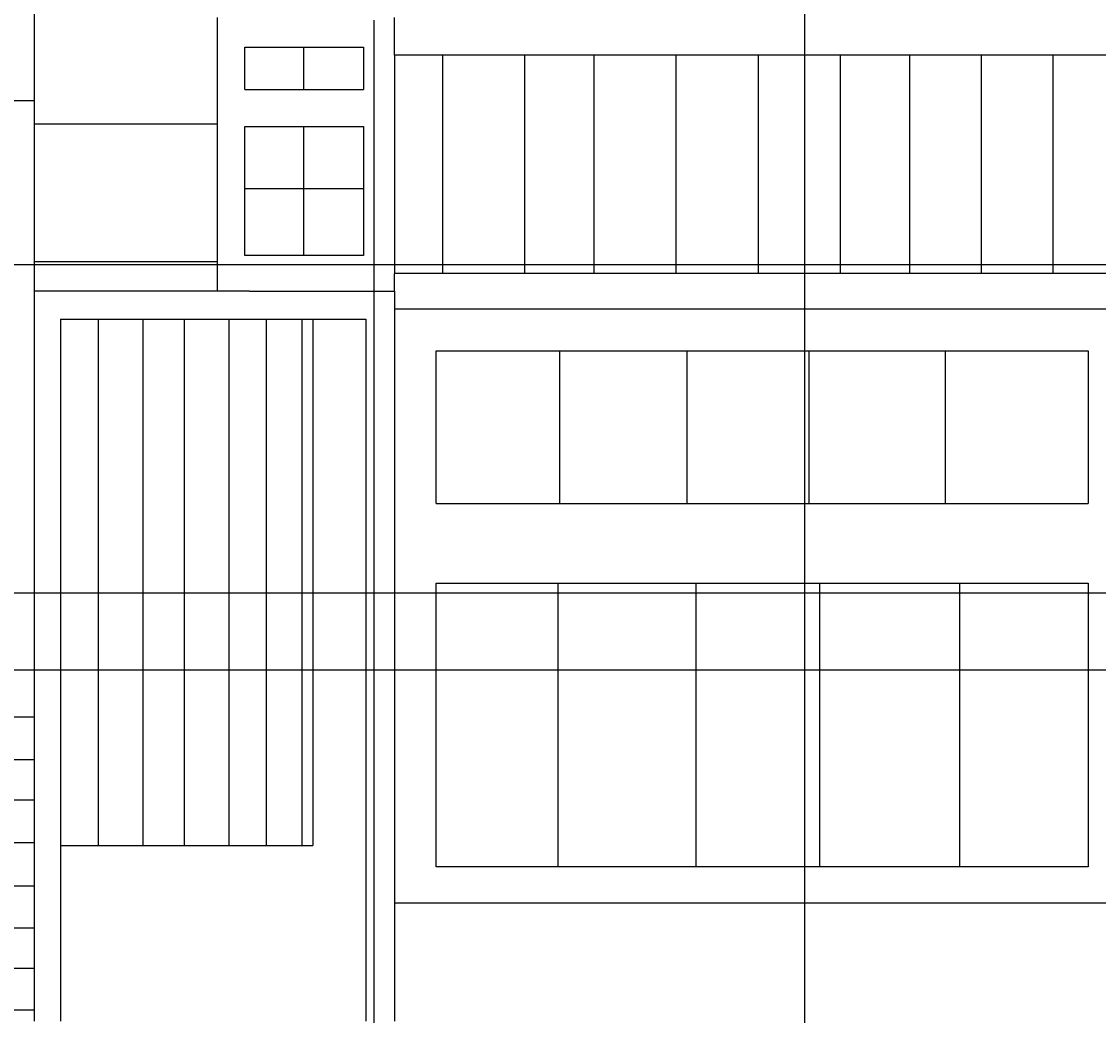
# Model space of a CAD drawing. Units: inches. Extents: x -117 to 121, y -77 to 40.
# Tile 21 of 45: x -23 to 3, y -32 to -8. Entities that reach past the tile are written whole.
import ezdxf

# ---------------------------------------------------------------- set-up
doc = ezdxf.new("R2010")
doc.units = ezdxf.units.IN
doc.header["$MEASUREMENT"] = 0
doc.layers.add('A-ANNO-DIMS', color=2, linetype='Continuous', lineweight=18)
doc.layers.add('A-ELEV', color=7, linetype='Continuous', lineweight=25)
doc.styles.get("Standard").update_dxf_attribs({"font": 'arial.ttf'})
doc.dimstyles.get("Standard").update_dxf_attribs({"dimtxt": 0.18, "dimasz": 0.18, "dimexe": 0.18, "dimexo": 0.0625, "dimgap": 0.09, "dimtad": 0, "dimtih": 1, "dimtoh": 1, "dimdec": 4, "dimzin": 0, "dimdsep": 46, "dimtxsty": 'Standard', "dimcen": 0.09, "dimadec": 0, "dimazin": 0, "dimtfac": 1, "dimtdec": 4, "dimtofl": 0, "dimtmove": 0, "dimatfit": 3, "dimfxl": 1, "dimtolj": 1, "dimtzin": 0, "dimarcsym": 0})

# ---------------------------------------------------------------- blocks, each defined once
blk = doc.blocks.new('*D13')
at = {"layer": 'A-ANNO-DIMS', "color": 0, "lineweight": -2, "transparency": 16777216}
for p, q in [((-2.663, 27.063), (-117.024, 27.063)), ((-116.844, 26.883), (-116.844, -16.974)), ((-116.844, -61.196), (-116.844, -17.338)), ((-106.096, -61.376), (-117.024, -61.376))]:
    blk.add_line(p, q, dxfattribs=at)
at = {"layer": 'A-ANNO-DIMS', "color": 0, "transparency": 16777216}
for points in [[(-116.874, 26.883), (-116.814, 26.883), (-116.844, 27.063)], [(-116.874, -61.196), (-116.814, -61.196), (-116.844, -61.376)]]:
    blk.add_solid(points, dxfattribs=at)
at = {"layer": 'Defpoints', "color": 0, "transparency": 16777216}
for p in [(-2.6, 27.063), (-116.844, -61.376), (-106.034, -61.376)]:
    blk.add_point(p, dxfattribs=at)
at = {"layer": 'A-ANNO-DIMS', "color": 0, "transparency": 16777216, "insert": (-116.844, -17.156), "char_height": 0.18, "attachment_point": 5}
blk.add_mtext('\\A1;88.44', dxfattribs=at)
blk = doc.blocks.new('*D32')
at = {"layer": 'A-ANNO-DIMS', "color": 0, "lineweight": -2, "transparency": 16777216}
for p, q in [((-3.85, -45.55), (-3.85, 38.61)), ((-3.67, 38.43), (7.757, 38.43)), ((20.113, 38.43), (8.686, 38.43)), ((20.293, -45.55), (20.293, 38.61))]:
    blk.add_line(p, q, dxfattribs=at)
at = {"layer": 'A-ANNO-DIMS', "color": 0, "transparency": 16777216}
for points in [[(-3.67, 38.46), (-3.67, 38.4), (-3.85, 38.43)], [(20.113, 38.46), (20.113, 38.4), (20.293, 38.43)]]:
    blk.add_solid(points, dxfattribs=at)
at = {"layer": 'Defpoints', "color": 0, "transparency": 16777216}
for p in [(20.293, 38.43), (-3.85, -45.613), (20.293, -45.613)]:
    blk.add_point(p, dxfattribs=at)
at = {"layer": 'A-ANNO-DIMS', "color": 0, "transparency": 16777216, "insert": (8.222, 38.43), "char_height": 0.18, "attachment_point": 5}
blk.add_mtext('\\A1;24.142', dxfattribs=at)
blk = doc.blocks.new('*D49')
at = {"layer": 'A-ANNO-DIMS', "color": 0, "lineweight": -2, "transparency": 16777216}
for p, q in [((-45.422, -23.501), (120.84, -23.501)), ((120.66, -23.681), (120.66, -31.426)), ((120.66, -39.536), (120.66, -31.79)), ((-45.471, -39.716), (120.84, -39.716))]:
    blk.add_line(p, q, dxfattribs=at)
at = {"layer": 'A-ANNO-DIMS', "color": 0, "transparency": 16777216}
for points in [[(120.63, -23.681), (120.69, -23.681), (120.66, -23.501)], [(120.63, -39.536), (120.69, -39.536), (120.66, -39.716)]]:
    blk.add_solid(points, dxfattribs=at)
at = {"layer": 'Defpoints', "color": 0, "transparency": 16777216}
for p in [(-45.485, -23.501), (120.66, -23.501), (-45.533, -39.716)]:
    blk.add_point(p, dxfattribs=at)
at = {"layer": 'A-ANNO-DIMS', "color": 0, "transparency": 16777216, "insert": (120.66, -31.608), "char_height": 0.18, "attachment_point": 5}
blk.add_mtext('\\A1;16.215', dxfattribs=at)
blk = doc.blocks.new('*D50')
at = {"layer": 'A-ANNO-DIMS', "color": 0, "lineweight": -2, "transparency": 16777216}
for p, q in [((-47.458, -13.74), (120.84, -13.74)), ((120.66, -13.92), (120.66, -17.512)), ((120.66, -21.468), (120.66, -17.876)), ((-47.458, -21.648), (120.84, -21.648))]:
    blk.add_line(p, q, dxfattribs=at)
at = {"layer": 'A-ANNO-DIMS', "color": 0, "transparency": 16777216}
for points in [[(120.63, -13.92), (120.69, -13.92), (120.66, -13.74)], [(120.63, -21.468), (120.69, -21.468), (120.66, -21.648)]]:
    blk.add_solid(points, dxfattribs=at)
at = {"layer": 'Defpoints', "color": 0, "transparency": 16777216}
for p in [(-47.521, -13.74), (120.66, -13.74), (-47.521, -21.648)]:
    blk.add_point(p, dxfattribs=at)
at = {"layer": 'A-ANNO-DIMS', "color": 0, "transparency": 16777216, "insert": (120.66, -17.694), "char_height": 0.18, "attachment_point": 5}
blk.add_mtext('\\A1;7.908', dxfattribs=at)
blk = doc.blocks.new('*D56')
at = {"layer": 'A-ANNO-DIMS', "color": 0, "lineweight": -2, "transparency": 16777216}
for p, q in [((-14.23, -7.853), (-14.23, -77.193)), ((7.628, -8.105), (7.628, -77.193)), ((-14.05, -77.013), (-3.766, -77.013)), ((7.448, -77.013), (-2.835, -77.013))]:
    blk.add_line(p, q, dxfattribs=at)
at = {"layer": 'A-ANNO-DIMS', "color": 0, "transparency": 16777216}
for points in [[(-14.05, -76.983), (-14.05, -77.043), (-14.23, -77.013)], [(7.448, -76.983), (7.448, -77.043), (7.628, -77.013)]]:
    blk.add_solid(points, dxfattribs=at)
at = {"layer": 'Defpoints', "color": 0, "transparency": 16777216}
for p in [(-14.23, -7.791), (7.628, -8.042), (7.628, -77.013)]:
    blk.add_point(p, dxfattribs=at)
at = {"layer": 'A-ANNO-DIMS', "color": 0, "transparency": 16777216, "insert": (-3.301, -77.013), "char_height": 0.18, "attachment_point": 5}
blk.add_mtext('\\A1;21.858', dxfattribs=at)

msp = doc.modelspace()

# ---------------------------------------------------------------- linework, layer by layer
at = {"layer": 'A-ELEV'}
for p, q in [((-22.4056, 14.0735), (-22.4056, -14.3771)), ((-18.0037, -7.7907), (-18.0037, -14.3771)), ((-13.7272, -8.6912), (-13.7272, -7.7907)), ((-17.3354, -8.4987), (-14.4795, -8.4987)), ((-17.3354, -9.5238), (-17.3354, -8.4987)), ((-15.9118, -9.5238), (-15.9118, -8.4987)), ((-14.4795, -8.4987), (-14.4795, -9.5238)), ((3.9947, -8.6912), (-13.7272, -8.6912)), ((-13.727, -13.9556), (-13.727, -8.6912)), ((-12.5711, -13.9556), (-12.5711, -8.6912)), ((-10.5946, -13.9556), (-10.5946, -8.6912)), ((-8.9222, -13.9556), (-8.9222, -8.6912)), ((-6.9457, -13.9556), (-6.9457, -8.6912)), ((-4.9691, -13.9556), (-4.9691, -8.6912)), ((-2.9926, -13.9556), (-2.9926, -8.6912)), ((-1.3202, -13.9556), (-1.3202, -8.6912)), ((0.4029, -13.9556), (0.4029, -8.6912)), ((2.1261, -13.9556), (2.1261, -8.6912)), ((-17.3354, -9.5238), (-14.4795, -9.5238)), ((-23.8637, -9.7904), (-22.4056, -9.7904)), ((-22.4056, -10.3496), (-18.0037, -10.3496)), ((-17.3354, -13.5225), (-17.3354, -10.4167)), ((-17.3354, -10.4167), (-14.4795, -10.4167)), ((-15.9118, -13.5225), (-15.9118, -10.4167)), ((-14.4795, -10.4167), (-14.4795, -13.5225)), ((-17.3354, -11.9047), (-14.4795, -11.9047)), ((-22.4056, -13.6676), (-18.0037, -13.6676)), ((-17.125, -13.5225), (-17.3354, -13.5225)), ((-14.4795, -13.5225), (-17.125, -13.5225)), ((-13.7366, -13.9556), (-13.7366, -14.3771)), ((3.9947, -13.9556), (-13.7272, -13.9556)), ((-17.2198, -14.3771), (-22.4056, -14.3771)), ((-22.4056, -14.3771), (-22.4056, -24.6358)), ((-17.2198, -14.3771), (-13.7272, -14.3771)), ((-13.7272, -14.3771), (-13.7272, -14.8161)), ((3.9947, -14.8161), (-13.7272, -14.8161)), ((-13.7272, -14.8161), (-13.7272, -29.1126)), ((-21.7693, -15.0526), (-14.4219, -15.0526)), ((-21.7693, -15.0526), (-21.7693, -31.9617)), ((-20.8693, -15.0526), (-20.8693, -27.7345)), ((-19.7893, -15.0526), (-19.7893, -27.7345)), ((-18.7993, -15.0526), (-18.7993, -27.7345)), ((-17.7193, -15.0526), (-17.7193, -27.7345)), ((-16.8193, -15.0526), (-16.8193, -27.7345)), ((-15.9643, -15.0526), (-15.9643, -27.7345)), ((-15.6943, -15.0526), (-15.6943, -27.7345)), ((-14.4219, -15.0526), (-14.4219, -31.9617)), ((-12.7273, -15.8183), (2.9753, -15.8183)), ((-12.7273, -19.4926), (-12.7273, -15.8183)), ((-9.7493, -19.4926), (-9.7493, -15.8183)), ((-6.6837, -19.4926), (-6.6837, -15.8183)), ((-3.7495, -19.4926), (-3.7495, -15.8183)), ((-0.465, -19.4926), (-0.465, -15.8183)), ((2.9753, -15.8183), (2.9753, -19.4926)), ((-12.7273, -19.4926), (2.9753, -19.4926)), ((-12.7273, -28.2437), (-12.7273, -21.4172)), ((-12.7273, -21.4172), (2.9753, -21.4172)), ((-9.7931, -28.2437), (-9.7931, -21.4172)), ((-6.4648, -28.2437), (-6.4648, -21.4172)), ((-3.4868, -28.2437), (-3.4868, -21.4172)), ((-0.1147, -28.2437), (-0.1147, -21.4172)), ((2.9753, -21.4172), (2.9753, -28.2437)), ((-45.4848, -24.6358), (-22.4056, -24.6358)), ((-22.4056, -24.6358), (-22.4056, -31.9617)), ((-27.6644, -25.6636), (-22.4056, -25.6636)), ((-27.6644, -26.6347), (-22.4056, -26.6347)), ((-27.6644, -27.6597), (-22.4056, -27.6597)), ((-21.7693, -27.7345), (-15.6943, -27.7345)), ((2.9753, -28.2437), (-12.7273, -28.2437)), ((-27.6644, -28.7066), (-22.4056, -28.7066)), ((-13.7272, -29.1126), (3.9947, -29.1126)), ((-13.7272, -29.1126), (-13.7272, -31.9617)), ((-27.6644, -29.7137), (-22.4056, -29.7137)), ((-27.6644, -30.6848), (-22.4056, -30.6848)), ((-27.6644, -31.6918), (-22.4056, -31.6918))]:
    msp.add_line(p, q, dxfattribs=at)

# ---------------------------------------------------------------- dimensions: what is measured, and where the dimension line sits
at = {"layer": 'A-ANNO-DIMS'}
for base, p1, p2, picture, middle in [((20.2929, 38.4297), (-3.8495, -45.6125), (20.2929, -45.6125), '*D32', (8.2217, 38.4297)), ((7.6284, -77.0135), (-14.2298, -7.7907), (7.6284, -8.0421), '*D56', (-3.3007, -77.0135))]:
    dim = msp.add_linear_dim(base=base, p1=p1, p2=p2, dimstyle='Standard', override={"dimdec": 3, "dimlfac": 1, "dimrnd": 0, "dimzin": 0, "dimdsep": 46, "dimlunit": 2}, dxfattribs=at)
    dim.commit()
    dim.dimension.update_dxf_attribs({"geometry": picture, "text_midpoint": middle})
for base, p1, p2, override, picture, middle in [((-116.8438, -61.3756), (-2.6001, 27.0634), (-106.0338, -61.3756), {"dimdec": 2, "dimlfac": 1, "dimrnd": 0, "dimzin": 0, "dimdsep": 46, "dimlunit": 2}, '*D13', (-116.8438, -17.1561)), ((120.6602, -13.74), (-47.5206, -21.6476), (-47.5206, -13.74), {"dimdec": 3, "dimlfac": 1, "dimrnd": 0, "dimzin": 0, "dimdsep": 46, "dimlunit": 2}, '*D50', (120.6602, -17.6938)), ((120.6602, -23.5007), (-45.5331, -39.716), (-45.4848, -23.5007), {"dimdec": 3, "dimlfac": 1, "dimrnd": 0, "dimzin": 0, "dimdsep": 46, "dimlunit": 2}, '*D49', (120.6602, -31.6083))]:
    dim = msp.add_linear_dim(base=base, p1=p1, p2=p2, angle=90, dimstyle='Standard', override=override, dxfattribs=at)
    dim.commit()
    dim.dimension.update_dxf_attribs({"geometry": picture, "text_midpoint": middle})

doc.saveas('drawing.dxf')
